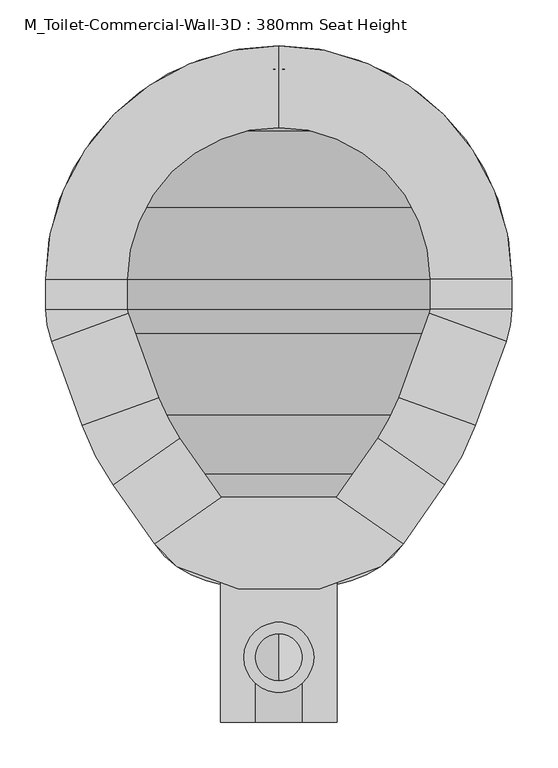
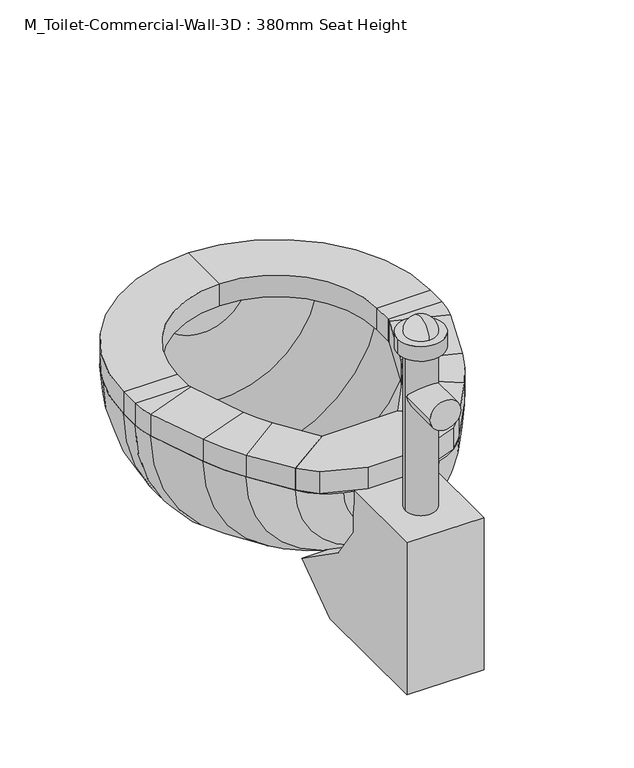
"""IFC4 building model written with IfcOpenShell, lengths in millimetres: flow terminal geometry, M_Toilet-Commercial-Wall-3D : 380mm Seat Height."""

from ifc_helpers import new_model, si_unit, point, frame, frame_2d, origin, place, context, project, spatial, polyline, circle_curve, ellipse_curve, trimmed, segment, composite_curve, outline, extrude, source, transform, mapped, element, save
from ifc_brep_helpers import plane_surface, cylinder_surface, revolved_surface, advanced_brep


def m_toilet_commercial_wall_3d_380mm_seat_height_fb359b30(model_context):
    return source(origin(), model_context, "Body", "SolidModel", [
        extrude(outline(polyline([(227.8037941, 341.9), (227.8037941, 268.296452), (271.5103185, 205.8770663), (375.5426282, 133.0328588), (295.0454017, 76.2), (75.0, 76.2), (75.0, 341.9), (227.8037941, 341.9)])), frame((341.4031538, 0.0, 0.0), z_axis=(1.0, 0.0, 0.0), x_axis=(0.0, 1.0, 0.0)), (0.0, 0.0, 1.0), 127.0),
        extrude(outline(composite_curve([segment(trimmed(circle_curve(frame_2d((404.9031538, 145.5352737)), 25.4), [point((379.5031538, 145.5352737))], [point((430.3031538, 145.5352737))], False, "CARTESIAN"), True, "CONTINUOUS"), segment(trimmed(circle_curve(frame_2d((404.9031538, 145.5352737)), 25.4), [point((430.3031538, 145.5352737))], [point((379.5031538, 145.5352737))], False, "CARTESIAN"), True, "CONTINUOUS")], self_intersect=False)), frame((0.0, 0.0, 341.9), z_axis=(0.0, 0.0, 1.0), x_axis=(1.0, 0.0, 0.0)), (0.0, 0.0, 1.0), 279.4),
        extrude(outline(composite_curve([segment(trimmed(circle_curve(frame_2d((543.2113641, 404.9031538)), 25.4), [point((543.2113641, 379.5031538))], [point((543.2113641, 430.3031538))], False, "CARTESIAN"), True, "CONTINUOUS"), segment(trimmed(circle_curve(frame_2d((543.2113641, 404.9031538)), 25.4), [point((543.2113641, 430.3031538))], [point((543.2113641, 379.5031538))], False, "CARTESIAN"), True, "CONTINUOUS")], self_intersect=False)), frame((0.0, 75.0, 0.0), z_axis=(0.0, 1.0, 0.0), x_axis=(0.0, 0.0, 1.0)), (0.0, 0.0, 1.0), 70.64375),
        extrude(outline(composite_curve([segment(trimmed(circle_curve(frame_2d((404.9031538, 145.5352737)), 38.1), [point((366.8031538, 145.5352737))], [point((443.0031538, 145.5352737))], False, "CARTESIAN"), True, "CONTINUOUS"), segment(trimmed(circle_curve(frame_2d((404.9031538, 145.5352737)), 38.1), [point((443.0031538, 145.5352737))], [point((366.8031538, 145.5352737))], False, "CARTESIAN"), True, "CONTINUOUS")], self_intersect=False)), frame((0.0, 0.0, 621.3), z_axis=(0.0, 0.0, 1.0), x_axis=(1.0, 0.0, 0.0)), (0.0, 0.0, 1.0), 25.4),
        advanced_brep(
        [(404.9031538, 119.9176912, 646.7), (404.9031538, 171.1528563, 646.7), (404.9031538, 145.5352737, 672.3175826), (404.9031538, 145.5352737, 646.7)],
        [
            (0, 1, circle_curve(frame((404.9031538, 145.5352737, 646.7), z_axis=(0.0, 0.0, 1.0), x_axis=(0.0, 1.0, 0.0)), 25.6175826)),
            (1, 2, circle_curve(frame((404.9031538, 145.5352737, 646.7), z_axis=(1.0, 0.0, 0.0), x_axis=(0.0, -1.0, 0.0)), 25.6175826)),
            (2, 0, circle_curve(frame((404.9031538, 145.5352737, 646.7), z_axis=(1.0, 0.0, 0.0), x_axis=(0.0, 1.0, 0.0)), 25.6175826)),
            (1, 0, circle_curve(frame((404.9031538, 145.5352737, 646.7), z_axis=(0.0, 0.0, 1.0), x_axis=(0.0, 1.0, 0.0)), 25.6175826)),
            (3, 1),
            (0, 3),
        ],
        [
            revolved_surface(trimmed(ellipse_curve(frame((404.9031538, 145.5352737, 646.7), z_axis=(-1.0, 0.0, 0.0), x_axis=(0.0, -1.0, 0.0)), 25.6175826, 25.6175826), [point((404.9031538, 145.5352737, 672.3175826))], [point((404.9031538, 171.1528563, 646.7))], True, "CARTESIAN"), (404.9031538, 145.5352737, 711.3277273), (0.0, 0.0, -1.0)),
            plane_surface(frame((404.9031538, 145.5352737, 646.7), z_axis=(0.0, 0.0, -1.0), x_axis=(0.0, 1.0, 0.0))),
        ],
        [
            (0, [[1, 2, 3]]),
            (0, [[4, -3, -2]]),
            (1, [[5, -1, 6]]),
            (1, [[-6, -4, -5]]),
        ],
    ),
        advanced_brep(
        [(491.7762702, 796.2819257, 341.9), (404.9031538, 811.6, 341.9), (404.9031538, 786.2, 341.9), (483.0889586, 772.4137331, 341.9), (566.547764, 719.2446102, 341.9), (619.7168869, 635.7858048, 341.9), (633.5031538, 557.6, 341.9), (633.5031538, 524.7148212, 341.9), (628.9077315, 498.6528863, 341.9), (596.6355667, 409.9858422, 341.9), (562.9565296, 345.2890139, 341.9), (525.0728964, 291.1855786, 341.9), (468.1430637, 251.3228806, 341.9), (404.9031538, 234.3777978, 341.9), (404.9031538, 208.0817829, 341.9), (483.6469009, 229.1811063, 341.9), (540.5767337, 269.0438043, 341.9), (585.6810159, 333.4593951, 341.9), (619.360053, 398.1562234, 341.9), (652.7759241, 489.9655747, 341.9), (658.9031538, 524.7148212, 341.9), (658.9031538, 557.6, 341.9), (643.5850795, 644.4731164, 341.9), (584.5082762, 737.2051224, 341.9), (318.0300374, 796.2819257, 341.9), (225.2980314, 737.2051224, 341.9), (166.2212281, 644.4731164, 341.9), (150.9031538, 557.6, 341.9), (150.9031538, 524.7148212, 341.9), (157.0303835, 489.9655747, 341.9), (190.4462546, 398.1562234, 341.9), (224.1252917, 333.4593951, 341.9), (269.229574, 269.0438043, 341.9), (326.1594067, 229.1811063, 341.9), (341.663244, 251.3228806, 341.9), (284.7334112, 291.1855786, 341.9), (246.849778, 345.2890139, 341.9), (213.1707409, 409.9858422, 341.9), (180.8985761, 498.6528863, 341.9), (176.3031538, 524.7148212, 341.9), (176.3031538, 557.6, 341.9), (190.0894207, 635.7858048, 341.9), (243.2585436, 719.2446102, 341.9), (326.7173491, 772.4137331, 341.9)],
        [
            (0, 1, circle_curve(frame((404.9031538, 557.6, 341.9), z_axis=(0.0, 0.0, 1.0), x_axis=(1.0, 0.0, 0.0)), 254.0)),
            (1, 2),
            (2, 3, circle_curve(frame((404.9031538, 557.6, 341.9), z_axis=(0.0, 0.0, -1.0), x_axis=(1.0, 0.0, 0.0)), 228.6)),
            (3, 4, circle_curve(frame((404.9031538, 557.6, 341.9), z_axis=(0.0, 0.0, -1.0), x_axis=(1.0, 0.0, 0.0)), 228.6)),
            (4, 5, circle_curve(frame((404.9031538, 557.6, 341.9), z_axis=(0.0, 0.0, -1.0), x_axis=(1.0, 0.0, 0.0)), 228.6)),
            (5, 6, circle_curve(frame((404.9031538, 557.6, 341.9), z_axis=(0.0, 0.0, -1.0), x_axis=(1.0, 0.0, 0.0)), 228.6)),
            (6, 7),
            (7, 8, circle_curve(frame((557.3031538, 524.7148212, 341.9), z_axis=(0.0, 0.0, -1.0), x_axis=(1.0, 0.0, 0.0)), 76.2)),
            (8, 9),
            (9, 10, circle_curve(frame((334.0854485, 505.5462703, 341.9), z_axis=(0.0, 0.0, -1.0), x_axis=(1.0, 0.0, 0.0)), 279.4)),
            (10, 11),
            (11, 12, circle_curve(frame((441.8470487, 349.4609446, 341.9), z_axis=(0.0, 0.0, -1.0), x_axis=(1.0, 0.0, 0.0)), 101.6)),
            (12, 13),
            (13, 14),
            (14, 15),
            (15, 16, circle_curve(frame((457.350886, 327.3191703, 341.9), z_axis=(0.0, 0.0, 1.0), x_axis=(1.0, 0.0, 0.0)), 101.6)),
            (16, 17),
            (17, 18, circle_curve(frame((356.8099347, 493.7166514, 341.9), z_axis=(0.0, 0.0, 1.0), x_axis=(1.0, 0.0, 0.0)), 279.4)),
            (18, 19),
            (19, 20, circle_curve(frame((557.3031538, 524.7148212, 341.9), z_axis=(0.0, 0.0, 1.0), x_axis=(1.0, 0.0, 0.0)), 101.6)),
            (20, 21),
            (21, 22, circle_curve(frame((404.9031538, 557.6, 341.9), z_axis=(0.0, 0.0, 1.0), x_axis=(1.0, 0.0, 0.0)), 254.0)),
            (22, 23, circle_curve(frame((404.9031538, 557.6, 341.9), z_axis=(0.0, 0.0, 1.0), x_axis=(1.0, 0.0, 0.0)), 254.0)),
            (23, 0, circle_curve(frame((404.9031538, 557.6, 341.9), z_axis=(0.0, 0.0, 1.0), x_axis=(1.0, 0.0, 0.0)), 254.0)),
            (24, 25, circle_curve(frame((404.9031538, 557.6, 341.9), z_axis=(0.0, 0.0, 1.0), x_axis=(-1.0, 0.0, 0.0)), 254.0)),
            (25, 26, circle_curve(frame((404.9031538, 557.6, 341.9), z_axis=(0.0, 0.0, 1.0), x_axis=(-1.0, 0.0, 0.0)), 254.0)),
            (26, 27, circle_curve(frame((404.9031538, 557.6, 341.9), z_axis=(0.0, 0.0, 1.0), x_axis=(-1.0, 0.0, 0.0)), 254.0)),
            (27, 28),
            (28, 29, circle_curve(frame((252.5031538, 524.7148212, 341.9), z_axis=(0.0, 0.0, 1.0), x_axis=(-1.0, 0.0, 0.0)), 101.6)),
            (29, 30),
            (30, 31, circle_curve(frame((452.9963729, 493.7166514, 341.9), z_axis=(0.0, 0.0, 1.0), x_axis=(-1.0, 0.0, 0.0)), 279.4)),
            (31, 32),
            (32, 33, circle_curve(frame((352.4554217, 327.3191703, 341.9), z_axis=(0.0, 0.0, 1.0), x_axis=(-1.0, 0.0, 0.0)), 101.6)),
            (33, 14),
            (13, 34),
            (34, 35, circle_curve(frame((367.9592589, 349.4609446, 341.9), z_axis=(0.0, 0.0, -1.0), x_axis=(-1.0, 0.0, 0.0)), 101.6)),
            (35, 36),
            (36, 37, circle_curve(frame((475.7208592, 505.5462703, 341.9), z_axis=(0.0, 0.0, -1.0), x_axis=(-1.0, 0.0, 0.0)), 279.4)),
            (37, 38),
            (38, 39, circle_curve(frame((252.5031538, 524.7148212, 341.9), z_axis=(0.0, 0.0, -1.0), x_axis=(-1.0, 0.0, 0.0)), 76.2)),
            (39, 40),
            (40, 41, circle_curve(frame((404.9031538, 557.6, 341.9), z_axis=(0.0, 0.0, -1.0), x_axis=(-1.0, 0.0, 0.0)), 228.6)),
            (41, 42, circle_curve(frame((404.9031538, 557.6, 341.9), z_axis=(0.0, 0.0, -1.0), x_axis=(-1.0, 0.0, 0.0)), 228.6)),
            (42, 43, circle_curve(frame((404.9031538, 557.6, 341.9), z_axis=(0.0, 0.0, -1.0), x_axis=(-1.0, 0.0, 0.0)), 228.6)),
            (43, 2, circle_curve(frame((404.9031538, 557.6, 341.9), z_axis=(0.0, 0.0, -1.0), x_axis=(-1.0, 0.0, 0.0)), 228.6)),
            (1, 24, circle_curve(frame((404.9031538, 557.6, 341.9), z_axis=(0.0, 0.0, 1.0), x_axis=(-1.0, 0.0, 0.0)), 254.0)),
            (0, 24, circle_curve(frame((404.9031538, 796.2819257, 341.9), z_axis=(0.0, 1.0, 0.0), x_axis=(1.0, 0.0, 0.0)), 86.8731164)),
            (43, 3, circle_curve(frame((404.9031538, 772.4137331, 341.9), z_axis=(0.0, -1.0, 0.0), x_axis=(1.0, 0.0, 0.0)), 78.1858048)),
            (42, 4, circle_curve(frame((404.9031538, 719.2446102, 341.9), z_axis=(0.0, -1.0, 0.0), x_axis=(1.0, 0.0, 0.0)), 161.6446102)),
            (41, 5, circle_curve(frame((404.9031538, 635.7858048, 341.9), z_axis=(0.0, -1.0, 0.0), x_axis=(1.0, 0.0, 0.0)), 214.8137331)),
            (40, 6, circle_curve(frame((404.9031538, 557.6, 341.9), z_axis=(0.0, -1.0, 0.0), x_axis=(1.0, 0.0, 0.0)), 228.6)),
            (39, 7, circle_curve(frame((404.9031538, 524.7148212, 341.9), z_axis=(0.0, -1.0, 0.0), x_axis=(1.0, 0.0, 0.0)), 228.6)),
            (38, 8, circle_curve(frame((404.9031538, 498.6528863, 341.9), z_axis=(0.0, -1.0, 0.0), x_axis=(1.0, 0.0, 0.0)), 224.0045777)),
            (37, 9, circle_curve(frame((404.9031538, 409.9858422, 341.9), z_axis=(0.0, -1.0, 0.0), x_axis=(1.0, 0.0, 0.0)), 191.7324129)),
            (36, 10, circle_curve(frame((404.9031538, 345.2890139, 341.9), z_axis=(0.0, -1.0, 0.0), x_axis=(1.0, 0.0, 0.0)), 158.0533758)),
            (35, 11, circle_curve(frame((404.9031538, 291.1855786, 341.9), z_axis=(0.0, -1.0, 0.0), x_axis=(1.0, 0.0, 0.0)), 120.1697426)),
            (34, 12, circle_curve(frame((404.9031538, 251.3228806, 341.9), z_axis=(0.0, -1.0, 0.0), x_axis=(1.0, 0.0, 0.0)), 63.2399099)),
            (33, 15, circle_curve(frame((404.9031538, 229.1811063, 341.9), z_axis=(0.0, -1.0, 0.0), x_axis=(1.0, 0.0, 0.0)), 78.7437471)),
            (32, 16, circle_curve(frame((404.9031538, 269.0438043, 341.9), z_axis=(0.0, -1.0, 0.0), x_axis=(1.0, 0.0, 0.0)), 135.6735798)),
            (31, 17, circle_curve(frame((404.9031538, 333.4593951, 341.9), z_axis=(0.0, -1.0, 0.0), x_axis=(1.0, 0.0, 0.0)), 180.7778621)),
            (30, 18, circle_curve(frame((404.9031538, 398.1562234, 341.9), z_axis=(0.0, -1.0, 0.0), x_axis=(1.0, 0.0, 0.0)), 214.4568992)),
            (29, 19, circle_curve(frame((404.9031538, 489.9655747, 341.9), z_axis=(0.0, -1.0, 0.0), x_axis=(1.0, 0.0, 0.0)), 247.8727703)),
            (28, 20, circle_curve(frame((404.9031538, 524.7148212, 341.9), z_axis=(0.0, -1.0, 0.0), x_axis=(1.0, 0.0, 0.0)), 254.0)),
            (27, 21, circle_curve(frame((404.9031538, 557.6, 341.9), z_axis=(0.0, -1.0, 0.0), x_axis=(1.0, 0.0, 0.0)), 254.0)),
            (26, 22, circle_curve(frame((404.9031538, 644.4731164, 341.9), z_axis=(0.0, -1.0, 0.0), x_axis=(1.0, 0.0, 0.0)), 238.6819257)),
            (25, 23, circle_curve(frame((404.9031538, 737.2051224, 341.9), z_axis=(0.0, -1.0, 0.0), x_axis=(1.0, 0.0, 0.0)), 179.6051224)),
        ],
        [
            plane_surface(frame((404.9031538, 916.8102448, 341.9), z_axis=(0.0, 0.0, 1.0), x_axis=(1.0, 0.0, 0.0))),
            plane_surface(frame((404.9031538, 916.8102448, 341.9), z_axis=(0.0, 0.0, 1.0), x_axis=(-1.0, 0.0, 0.0))),
            revolved_surface(trimmed(ellipse_curve(frame((404.9031538, 557.6, 341.9), z_axis=(0.0, 0.0, 1.0), x_axis=(1.0, 0.0, 0.0)), 254.0, 254.0), [point((491.7762702, 796.2819257, 341.9))], [point((404.9031538, 811.6, 341.9))], True, "CARTESIAN"), (404.9031538, 916.8102448, 341.9), (0.0, 1.0, 0.0)),
            revolved_surface(trimmed(ellipse_curve(frame((404.9031538, 557.6, 341.9), z_axis=(0.0, 0.0, -1.0), x_axis=(1.0, 0.0, 0.0)), 228.6, 228.6), [point((404.9031538, 786.2, 341.9))], [point((483.0889586, 772.4137331, 341.9))], True, "CARTESIAN"), (404.9031538, 916.8102448, 341.9), (0.0, 1.0, 0.0)),
            revolved_surface(trimmed(ellipse_curve(frame((404.9031538, 557.6, 341.9), z_axis=(0.0, 0.0, -1.0), x_axis=(1.0, 0.0, 0.0)), 228.6, 228.6), [point((483.0889586, 772.4137331, 341.9))], [point((566.547764, 719.2446102, 341.9))], True, "CARTESIAN"), (404.9031538, 916.8102448, 341.9), (0.0, 1.0, 0.0)),
            revolved_surface(trimmed(ellipse_curve(frame((404.9031538, 557.6, 341.9), z_axis=(0.0, 0.0, -1.0), x_axis=(1.0, 0.0, 0.0)), 228.6, 228.6), [point((566.547764, 719.2446102, 341.9))], [point((619.7168869, 635.7858048, 341.9))], True, "CARTESIAN"), (404.9031538, 916.8102448, 341.9), (0.0, 1.0, 0.0)),
            revolved_surface(trimmed(ellipse_curve(frame((404.9031538, 557.6, 341.9), z_axis=(0.0, 0.0, -1.0), x_axis=(1.0, 0.0, 0.0)), 228.6, 228.6), [point((619.7168869, 635.7858048, 341.9))], [point((633.5031538, 557.6, 341.9))], True, "CARTESIAN"), (404.9031538, 916.8102448, 341.9), (0.0, 1.0, 0.0)),
            revolved_surface(polyline([(633.5031538, 557.6, 341.9), (633.5031538, 524.7148212, 341.9)]), (404.9031538, 916.8102448, 341.9), (0.0, 1.0, 0.0)),
            revolved_surface(trimmed(ellipse_curve(frame((557.3031538, 524.7148212, 341.9), z_axis=(0.0, 0.0, -1.0), x_axis=(1.0, 0.0, 0.0)), 76.2, 76.2), [point((633.5031538, 524.7148212, 341.9))], [point((628.9077315, 498.6528863, 341.9))], True, "CARTESIAN"), (404.9031538, 916.8102448, 341.9), (0.0, 1.0, 0.0)),
            revolved_surface(polyline([(628.9077315, 498.6528863, 341.9), (596.6355667, 409.9858422, 341.9)]), (404.9031538, 916.8102448, 341.9), (0.0, 1.0, 0.0)),
            revolved_surface(trimmed(ellipse_curve(frame((334.0854485, 505.5462703, 341.9), z_axis=(0.0, 0.0, -1.0), x_axis=(1.0, 0.0, 0.0)), 279.4, 279.4), [point((596.6355667, 409.9858422, 341.9))], [point((562.9565296, 345.2890139, 341.9))], True, "CARTESIAN"), (404.9031538, 916.8102448, 341.9), (0.0, 1.0, 0.0)),
            revolved_surface(polyline([(562.9565296, 345.2890139, 341.9), (525.0728964, 291.1855786, 341.9)]), (404.9031538, 916.8102448, 341.9), (0.0, 1.0, 0.0)),
            revolved_surface(trimmed(ellipse_curve(frame((441.8470487, 349.4609446, 341.9), z_axis=(0.0, 0.0, -1.0), x_axis=(1.0, 0.0, 0.0)), 101.6, 101.6), [point((525.0728964, 291.1855786, 341.9))], [point((468.1430637, 251.3228806, 341.9))], True, "CARTESIAN"), (404.9031538, 916.8102448, 341.9), (0.0, 1.0, 0.0)),
            revolved_surface(polyline([(468.1430637, 251.3228806, 341.9), (404.9031538, 234.3777978, 341.9)]), (404.9031538, 916.8102448, 341.9), (0.0, 1.0, 0.0)),
            revolved_surface(polyline([(404.9031538, 208.0817829, 341.9), (483.6469009, 229.1811063, 341.9)]), (404.9031538, 916.8102448, 341.9), (0.0, 1.0, 0.0)),
            revolved_surface(trimmed(ellipse_curve(frame((457.350886, 327.3191703, 341.9), z_axis=(0.0, 0.0, 1.0), x_axis=(1.0, 0.0, 0.0)), 101.6, 101.6), [point((483.6469009, 229.1811063, 341.9))], [point((540.5767337, 269.0438043, 341.9))], True, "CARTESIAN"), (404.9031538, 916.8102448, 341.9), (0.0, 1.0, 0.0)),
            revolved_surface(polyline([(540.5767337, 269.0438043, 341.9), (585.6810159, 333.4593951, 341.9)]), (404.9031538, 916.8102448, 341.9), (0.0, 1.0, 0.0)),
            revolved_surface(trimmed(ellipse_curve(frame((356.8099347, 493.7166514, 341.9), z_axis=(0.0, 0.0, 1.0), x_axis=(1.0, 0.0, 0.0)), 279.4, 279.4), [point((585.6810159, 333.4593951, 341.9))], [point((619.360053, 398.1562234, 341.9))], True, "CARTESIAN"), (404.9031538, 916.8102448, 341.9), (0.0, 1.0, 0.0)),
            revolved_surface(polyline([(619.360053, 398.1562234, 341.9), (652.7759241, 489.9655747, 341.9)]), (404.9031538, 916.8102448, 341.9), (0.0, 1.0, 0.0)),
            revolved_surface(trimmed(ellipse_curve(frame((557.3031538, 524.7148212, 341.9), z_axis=(0.0, 0.0, 1.0), x_axis=(1.0, 0.0, 0.0)), 101.6, 101.6), [point((652.7759241, 489.9655747, 341.9))], [point((658.9031538, 524.7148212, 341.9))], True, "CARTESIAN"), (404.9031538, 916.8102448, 341.9), (0.0, 1.0, 0.0)),
            cylinder_surface(frame((404.9031538, 916.8102448, 341.9), z_axis=(0.0, 1.0, 0.0), x_axis=(1.0, 0.0, 0.0)), 254.0),
            revolved_surface(trimmed(ellipse_curve(frame((404.9031538, 557.6, 341.9), z_axis=(0.0, 0.0, 1.0), x_axis=(1.0, 0.0, 0.0)), 254.0, 254.0), [point((658.9031538, 557.6, 341.9))], [point((643.5850795, 644.4731164, 341.9))], True, "CARTESIAN"), (404.9031538, 916.8102448, 341.9), (0.0, 1.0, 0.0)),
            revolved_surface(trimmed(ellipse_curve(frame((404.9031538, 557.6, 341.9), z_axis=(0.0, 0.0, 1.0), x_axis=(1.0, 0.0, 0.0)), 254.0, 254.0), [point((643.5850795, 644.4731164, 341.9))], [point((584.5082762, 737.2051224, 341.9))], True, "CARTESIAN"), (404.9031538, 916.8102448, 341.9), (0.0, 1.0, 0.0)),
            revolved_surface(trimmed(ellipse_curve(frame((404.9031538, 557.6, 341.9), z_axis=(0.0, 0.0, 1.0), x_axis=(1.0, 0.0, 0.0)), 254.0, 254.0), [point((584.5082762, 737.2051224, 341.9))], [point((491.7762702, 796.2819257, 341.9))], True, "CARTESIAN"), (404.9031538, 916.8102448, 341.9), (0.0, 1.0, 0.0)),
        ],
        [
            (0, [[1, 2, 3, 4, 5, 6, 7, 8, 9, 10, 11, 12, 13, 14, 15, 16, 17, 18, 19, 20, 21, 22, 23, 24]]),
            (1, [[25, 26, 27, 28, 29, 30, 31, 32, 33, 34, -14, 35, 36, 37, 38, 39, 40, 41, 42, 43, 44, 45, -2, 46]]),
            (2, [[-1, 47, -46]]),
            (3, [[48, -3, -45]]),
            (4, [[49, -4, -48, -44]]),
            (5, [[50, -5, -49, -43]]),
            (6, [[51, -6, -50, -42]]),
            (7, [[52, -7, -51, -41]]),
            (8, [[53, -8, -52, -40]]),
            (9, [[54, -9, -53, -39]]),
            (10, [[55, -10, -54, -38]]),
            (11, [[56, -11, -55, -37]]),
            (12, [[57, -12, -56, -36]]),
            (13, [[-13, -57, -35]]),
            (14, [[58, -15, -34]]),
            (15, [[59, -16, -58, -33]]),
            (16, [[60, -17, -59, -32]]),
            (17, [[61, -18, -60, -31]]),
            (18, [[62, -19, -61, -30]]),
            (19, [[63, -20, -62, -29]]),
            (20, [[64, -21, -63, -28]]),
            (21, [[65, -22, -64, -27]]),
            (22, [[66, -23, -65, -26]]),
            (23, [[-47, -24, -66, -25]]),
        ],
    ),
        advanced_brep(
        [(467.7541169, 320.0347495, 341.9), (540.5767337, 269.0438043, 341.9), (540.5767337, 269.0438043, 380.0), (467.7541169, 320.0347495, 380.0), (512.8583992, 384.4503403, 341.9), (585.6810159, 333.4593951, 341.9), (585.6810159, 333.4593951, 380.0), (512.8583992, 384.4503403, 380.0), (619.360053, 398.1562234, 341.9), (535.821379, 428.5618141, 341.9), (619.360053, 398.1562234, 380.0), (535.821379, 428.5618141, 380.0), (569.2372501, 520.3711654, 341.9), (652.7759241, 489.9655747, 341.9), (652.7759241, 489.9655747, 380.0), (569.2372501, 520.3711654, 380.0), (658.9031538, 524.7148212, 341.9), (570.0031538, 524.7148212, 341.9), (658.9031538, 524.7148212, 380.0), (570.0031538, 524.7148212, 380.0), (570.0031538, 557.6, 341.9), (658.9031538, 557.6, 341.9), (658.9031538, 557.6, 380.0), (570.0031538, 557.6, 380.0), (404.9031538, 811.6, 341.9), (404.9031538, 722.7, 341.9), (404.9031538, 811.6, 380.0), (404.9031538, 722.7, 380.0), (150.9031538, 557.6, 341.9), (239.8031538, 557.6, 341.9), (150.9031538, 557.6, 380.0), (239.8031538, 557.6, 380.0), (239.8031538, 524.7148212, 341.9), (150.9031538, 524.7148212, 341.9), (150.9031538, 524.7148212, 380.0), (239.8031538, 524.7148212, 380.0), (157.0303835, 489.9655747, 341.9), (240.5690575, 520.3711654, 341.9), (157.0303835, 489.9655747, 380.0), (240.5690575, 520.3711654, 380.0), (273.9849286, 428.5618141, 341.9), (190.4462546, 398.1562234, 341.9), (190.4462546, 398.1562234, 380.0), (273.9849286, 428.5618141, 380.0), (224.1252917, 333.4593951, 341.9), (296.9479084, 384.4503403, 341.9), (224.1252917, 333.4593951, 380.0), (296.9479084, 384.4503403, 380.0), (342.0521907, 320.0347495, 341.9), (342.0521907, 320.0347495, 380.0), (269.229574, 269.0438043, 380.0), (269.229574, 269.0438043, 341.9)],
        [
            (0, 1),
            (1, 2),
            (2, 3),
            (3, 0),
            (0, 4),
            (4, 5),
            (5, 1),
            (5, 6),
            (6, 2),
            (6, 7),
            (7, 3),
            (7, 4),
            (8, 5, circle_curve(frame((356.8099347, 493.7166514, 341.9), z_axis=(0.0, 0.0, -1.0), x_axis=(0.819152044288991, -0.5735764363510472, 0.0)), 279.4)),
            (4, 9, circle_curve(frame((356.8099347, 493.7166514, 341.9), z_axis=(0.0, 0.0, 1.0), x_axis=(0.819152044288991, -0.5735764363510472, 0.0)), 190.5)),
            (9, 8),
            (10, 6, circle_curve(frame((356.8099347, 493.7166514, 380.0), z_axis=(0.0, 0.0, -1.0), x_axis=(0.819152044288991, -0.5735764363510472, 0.0)), 279.4)),
            (8, 10),
            (11, 7, circle_curve(frame((356.8099347, 493.7166514, 380.0), z_axis=(0.0, 0.0, -1.0), x_axis=(0.819152044288991, -0.5735764363510472, 0.0)), 190.5)),
            (10, 11),
            (11, 9),
            (9, 12),
            (12, 13),
            (13, 8),
            (13, 14),
            (14, 10),
            (14, 15),
            (15, 11),
            (15, 12),
            (16, 13, circle_curve(frame((557.3031538, 524.7148212, 341.9), z_axis=(0.0, 0.0, -1.0), x_axis=(0.93969262078591, -0.3420201433256644, 0.0)), 101.6)),
            (12, 17, circle_curve(frame((557.3031538, 524.7148212, 341.9), z_axis=(0.0, 0.0, 1.0), x_axis=(0.93969262078591, -0.3420201433256644, 0.0)), 12.7)),
            (17, 16),
            (18, 14, circle_curve(frame((557.3031538, 524.7148212, 380.0), z_axis=(0.0, 0.0, -1.0), x_axis=(0.93969262078591, -0.3420201433256644, 0.0)), 101.6)),
            (16, 18),
            (19, 15, circle_curve(frame((557.3031538, 524.7148212, 380.0), z_axis=(0.0, 0.0, -1.0), x_axis=(0.93969262078591, -0.3420201433256644, 0.0)), 12.7)),
            (18, 19),
            (19, 17),
            (17, 20),
            (20, 21),
            (21, 16),
            (21, 22),
            (22, 18),
            (22, 23),
            (23, 19),
            (23, 20),
            (24, 21, circle_curve(frame((404.9031538, 557.6, 341.9), z_axis=(0.0, 0.0, -1.0), x_axis=(1.0, 0.0, 0.0)), 254.0)),
            (20, 25, circle_curve(frame((404.9031538, 557.6, 341.9), z_axis=(0.0, 0.0, 1.0), x_axis=(1.0, 0.0, 0.0)), 165.1)),
            (25, 24),
            (26, 22, circle_curve(frame((404.9031538, 557.6, 380.0), z_axis=(0.0, 0.0, -1.0), x_axis=(1.0, 0.0, 0.0)), 254.0)),
            (24, 26),
            (27, 23, circle_curve(frame((404.9031538, 557.6, 380.0), z_axis=(0.0, 0.0, -1.0), x_axis=(1.0, 0.0, 0.0)), 165.1)),
            (26, 27),
            (27, 25),
            (28, 24, circle_curve(frame((404.9031538, 557.6, 341.9), z_axis=(0.0, 0.0, -1.0), x_axis=(0.0, 1.0, 0.0)), 254.0)),
            (25, 29, circle_curve(frame((404.9031538, 557.6, 341.9), z_axis=(0.0, 0.0, 1.0), x_axis=(0.0, 1.0, 0.0)), 165.1)),
            (29, 28),
            (30, 26, circle_curve(frame((404.9031538, 557.6, 380.0), z_axis=(0.0, 0.0, -1.0), x_axis=(0.0, 1.0, 0.0)), 254.0)),
            (28, 30),
            (31, 27, circle_curve(frame((404.9031538, 557.6, 380.0), z_axis=(0.0, 0.0, -1.0), x_axis=(0.0, 1.0, 0.0)), 165.1)),
            (30, 31),
            (31, 29),
            (29, 32),
            (32, 33),
            (33, 28),
            (33, 34),
            (34, 30),
            (34, 35),
            (35, 31),
            (35, 32),
            (36, 33, circle_curve(frame((252.5031538, 524.7148212, 341.9), z_axis=(0.0, 0.0, -1.0), x_axis=(-1.0, 0.0, 0.0)), 101.6)),
            (32, 37, circle_curve(frame((252.5031538, 524.7148212, 341.9), z_axis=(0.0, 0.0, 1.0), x_axis=(-1.0, 0.0, 0.0)), 12.7)),
            (37, 36),
            (38, 34, circle_curve(frame((252.5031538, 524.7148212, 380.0), z_axis=(0.0, 0.0, -1.0), x_axis=(-1.0, 0.0, 0.0)), 101.6)),
            (36, 38),
            (39, 35, circle_curve(frame((252.5031538, 524.7148212, 380.0), z_axis=(0.0, 0.0, -1.0), x_axis=(-1.0, 0.0, 0.0)), 12.7)),
            (38, 39),
            (39, 37),
            (37, 40),
            (40, 41),
            (41, 36),
            (41, 42),
            (42, 38),
            (42, 43),
            (43, 39),
            (43, 40),
            (44, 41, circle_curve(frame((452.9963729, 493.7166514, 341.9), z_axis=(0.0, 0.0, -1.0), x_axis=(-0.9396926207859084, -0.3420201433256685, 0.0)), 279.4)),
            (40, 45, circle_curve(frame((452.9963729, 493.7166514, 341.9), z_axis=(0.0, 0.0, 1.0), x_axis=(-0.9396926207859084, -0.3420201433256685, 0.0)), 190.5)),
            (45, 44),
            (46, 42, circle_curve(frame((452.9963729, 493.7166514, 380.0), z_axis=(0.0, 0.0, -1.0), x_axis=(-0.9396926207859084, -0.3420201433256685, 0.0)), 279.4)),
            (44, 46),
            (47, 43, circle_curve(frame((452.9963729, 493.7166514, 380.0), z_axis=(0.0, 0.0, -1.0), x_axis=(-0.9396926207859084, -0.3420201433256685, 0.0)), 190.5)),
            (46, 47),
            (47, 45),
            (48, 49),
            (49, 50),
            (50, 51),
            (51, 48),
            (45, 48),
            (51, 44),
            (50, 46),
            (49, 47),
        ],
        [
            plane_surface(frame((540.5767337, 269.0438043, 438.6203184), z_axis=(-0.5735764363510425, -0.8191520442889944, 0.0), x_axis=(0.8191520442889944, -0.5735764363510425, 0.0))),
            plane_surface(frame((467.7541169, 320.0347495, 341.9), z_axis=(0.0, 0.0, -1.0), x_axis=(0.5735764363510422, 0.8191520442889946, 0.0))),
            plane_surface(frame((540.5767337, 269.0438043, 341.9), z_axis=(0.8191520442889946, -0.5735764363510423, 0.0), x_axis=(0.5735764363510423, 0.8191520442889946, 0.0))),
            plane_surface(frame((540.5767337, 269.0438043, 380.0), z_axis=(0.0, 0.0, 1.0), x_axis=(0.5735764363510425, 0.8191520442889942, 0.0))),
            plane_surface(frame((467.7541169, 320.0347495, 380.0), z_axis=(-0.8191520442889942, 0.5735764363510425, 0.0), x_axis=(0.5735764363510425, 0.8191520442889942, 0.0))),
            plane_surface(frame((356.8099347, 493.7166514, 341.9), z_axis=(0.0, 0.0, -1.0), x_axis=(0.819152044288991, -0.5735764363510472, 0.0))),
            cylinder_surface(frame((356.8099347, 493.7166514, 341.9), z_axis=(0.0, 0.0, 1.0), x_axis=(0.819152044288991, -0.5735764363510472, 0.0)), 279.4),
            plane_surface(frame((356.8099347, 493.7166514, 380.0), z_axis=(0.0, 0.0, 1.0), x_axis=(0.819152044288991, -0.5735764363510472, 0.0))),
            revolved_surface(polyline([(512.8583991370527, 384.45034027512554, 380.0), (512.8583991370527, 384.45034027512554, 341.9)]), (356.8099347, 493.7166514, 341.9), (0.0, 0.0, 1.0)),
            plane_surface(frame((535.821379, 428.5618141, 341.9), z_axis=(0.0, 0.0, -1.0), x_axis=(0.34202014332565833, 0.9396926207859122, 0.0))),
            plane_surface(frame((619.360053, 398.1562234, 341.9), z_axis=(0.9396926207859126, -0.3420201433256572, 0.0), x_axis=(0.3420201433256572, 0.9396926207859126, 0.0))),
            plane_surface(frame((619.360053, 398.1562234, 380.0), z_axis=(0.0, 0.0, 1.0000000000000002), x_axis=(0.342020143325657, 0.9396926207859128, 0.0))),
            plane_surface(frame((535.821379, 428.5618141, 380.0), z_axis=(-0.9396926207859121, 0.342020143325659, 0.0), x_axis=(0.342020143325659, 0.9396926207859121, 0.0))),
            plane_surface(frame((557.3031538, 524.7148212, 341.9), z_axis=(0.0, 0.0, -1.0), x_axis=(0.93969262078591, -0.3420201433256644, 0.0))),
            cylinder_surface(frame((557.3031538, 524.7148212, 341.9), z_axis=(0.0, 0.0, 1.0), x_axis=(0.93969262078591, -0.3420201433256644, 0.0)), 101.6),
            plane_surface(frame((557.3031538, 524.7148212, 380.0), z_axis=(0.0, 0.0, 1.0), x_axis=(0.93969262078591, -0.3420201433256644, 0.0))),
            revolved_surface(polyline([(569.237250083981, 520.3711653797641, 380.0), (569.237250083981, 520.3711653797641, 341.9)]), (557.3031538, 524.7148212, 341.9), (0.0, 0.0, 1.0)),
            plane_surface(frame((570.0031538, 524.7148212, 341.9), z_axis=(0.0, 0.0, -1.0), x_axis=(0.0, 1.0, 0.0))),
            plane_surface(frame((658.9031538, 524.7148212, 341.9), z_axis=(1.0, 0.0, 0.0), x_axis=(0.0, 1.0, 0.0))),
            plane_surface(frame((658.9031538, 524.7148212, 380.0), z_axis=(0.0, 0.0, 1.0), x_axis=(0.0, 1.0, 0.0))),
            plane_surface(frame((570.0031538, 524.7148212, 380.0), z_axis=(-1.0, 0.0, 0.0), x_axis=(0.0, 1.0, 0.0))),
            plane_surface(frame((404.9031538, 557.6, 341.9), z_axis=(0.0, 0.0, -1.0), x_axis=(1.0, 0.0, 0.0))),
            cylinder_surface(frame((404.9031538, 557.6, 341.9), z_axis=(0.0, 0.0, 1.0), x_axis=(1.0, 0.0, 0.0)), 254.0),
            plane_surface(frame((404.9031538, 557.6, 380.0), z_axis=(0.0, 0.0, 1.0), x_axis=(1.0, 0.0, 0.0))),
            revolved_surface(polyline([(570.0031538, 557.6, 380.0), (570.0031538, 557.6, 341.9)]), (404.9031538, 557.6, 341.9), (0.0, 0.0, 1.0)),
            plane_surface(frame((404.9031538, 557.6, 341.9), z_axis=(0.0, 0.0, -1.0), x_axis=(0.0, 1.0, 0.0))),
            cylinder_surface(frame((404.9031538, 557.6, 341.9), z_axis=(0.0, 0.0, 1.0), x_axis=(0.0, 1.0, 0.0)), 254.0),
            plane_surface(frame((404.9031538, 557.6, 380.0), z_axis=(0.0, 0.0, 1.0), x_axis=(0.0, 1.0, 0.0))),
            revolved_surface(polyline([(404.9031538, 722.7, 380.0), (404.9031538, 722.7, 341.9)]), (404.9031538, 557.6, 341.9), (0.0, 0.0, 1.0)),
            plane_surface(frame((239.8031538, 557.6, 341.9), z_axis=(0.0, 0.0, -1.0), x_axis=(0.0, -1.0, 0.0))),
            plane_surface(frame((150.9031538, 557.6, 341.9), z_axis=(-1.0, 0.0, 0.0), x_axis=(0.0, -1.0, 0.0))),
            plane_surface(frame((150.9031538, 557.6, 380.0), z_axis=(0.0, 0.0, 1.0), x_axis=(0.0, -1.0, 0.0))),
            plane_surface(frame((239.8031538, 557.6, 380.0), z_axis=(1.0, 0.0, 0.0), x_axis=(0.0, -1.0, 0.0))),
            plane_surface(frame((252.5031538, 524.7148212, 341.9), z_axis=(0.0, 0.0, -1.0), x_axis=(-1.0, 0.0, 0.0))),
            cylinder_surface(frame((252.5031538, 524.7148212, 341.9), z_axis=(0.0, 0.0, 1.0), x_axis=(-1.0, 0.0, 0.0)), 101.6),
            plane_surface(frame((252.5031538, 524.7148212, 380.0), z_axis=(0.0, 0.0, 1.0), x_axis=(-1.0, 0.0, 0.0))),
            revolved_surface(polyline([(239.80315380000002, 524.7148212, 380.0), (239.80315380000002, 524.7148212, 341.9)]), (252.5031538, 524.7148212, 341.9), (0.0, 0.0, 1.0)),
            plane_surface(frame((240.5690575, 520.3711654, 341.9), z_axis=(0.0, 0.0, -1.0000000000000002), x_axis=(0.34202014332566893, -0.9396926207859084, 0.0))),
            plane_surface(frame((157.0303835, 489.9655747, 341.9), z_axis=(-0.9396926207859084, -0.3420201433256686, 0.0), x_axis=(0.3420201433256686, -0.9396926207859084, 0.0))),
            plane_surface(frame((157.0303835, 489.9655747, 380.0), z_axis=(0.0, 0.0, 1.0), x_axis=(0.3420201433256687, -0.9396926207859084, 0.0))),
            plane_surface(frame((240.5690575, 520.3711654, 380.0), z_axis=(0.9396926207859084, 0.3420201433256686, 0.0), x_axis=(0.3420201433256686, -0.9396926207859084, 0.0))),
            plane_surface(frame((452.9963729, 493.7166514, 341.9), z_axis=(0.0, 0.0, -1.0000000000000002), x_axis=(-0.9396926207859085, -0.34202014332566855, 0.0))),
            cylinder_surface(frame((452.9963729, 493.7166514, 341.9), z_axis=(0.0, 0.0, 1.0), x_axis=(-0.9396926207859084, -0.3420201433256685, 0.0)), 279.4),
            plane_surface(frame((452.9963729, 493.7166514, 380.0), z_axis=(0.0, 0.0, 1.0000000000000002), x_axis=(-0.9396926207859085, -0.34202014332566855, 0.0))),
            revolved_surface(polyline([(273.98492864028447, 428.5618140964601, 380.0), (273.98492864028447, 428.5618140964601, 341.9)]), (452.9963729, 493.7166514, 341.9), (0.0, 0.0, 1.0)),
            plane_surface(frame((269.229574, 269.0438043, 245.1796816), z_axis=(0.5735764363510472, -0.819152044288991, 0.0), x_axis=(0.819152044288991, 0.5735764363510472, 0.0))),
            plane_surface(frame((296.9479084, 384.4503403, 341.9), z_axis=(0.0, 0.0, -1.0), x_axis=(0.573576436351047, -0.8191520442889911, 0.0))),
            plane_surface(frame((224.1252917, 333.4593951, 341.9), z_axis=(-0.819152044288991, -0.5735764363510473, 0.0), x_axis=(0.5735764363510473, -0.819152044288991, 0.0))),
            plane_surface(frame((224.1252917, 333.4593951, 380.0), z_axis=(0.0, 0.0, 1.0), x_axis=(0.5735764363510477, -0.8191520442889907, 0.0))),
            plane_surface(frame((296.9479084, 384.4503403, 380.0), z_axis=(0.8191520442889914, 0.5735764363510468, 0.0), x_axis=(0.5735764363510468, -0.8191520442889914, 0.0))),
        ],
        [
            (0, [[1, 2, 3, 4]]),
            (1, [[-1, 5, 6, 7]]),
            (2, [[-2, -7, 8, 9]]),
            (3, [[-3, -9, 10, 11]]),
            (4, [[-4, -11, 12, -5]]),
            (5, [[13, -6, 14, 15]]),
            (6, [[16, -8, -13, 17]]),
            (7, [[18, -10, -16, 19]]),
            (8, [[-14, -12, -18, 20]]),
            (9, [[-15, 21, 22, 23]]),
            (10, [[-17, -23, 24, 25]]),
            (11, [[-19, -25, 26, 27]]),
            (12, [[-20, -27, 28, -21]]),
            (13, [[29, -22, 30, 31]]),
            (14, [[32, -24, -29, 33]]),
            (15, [[34, -26, -32, 35]]),
            (16, [[-30, -28, -34, 36]]),
            (17, [[-31, 37, 38, 39]]),
            (18, [[-33, -39, 40, 41]]),
            (19, [[-35, -41, 42, 43]]),
            (20, [[-36, -43, 44, -37]]),
            (21, [[45, -38, 46, 47]]),
            (22, [[48, -40, -45, 49]]),
            (23, [[50, -42, -48, 51]]),
            (24, [[-46, -44, -50, 52]]),
            (25, [[53, -47, 54, 55]]),
            (26, [[56, -49, -53, 57]]),
            (27, [[58, -51, -56, 59]]),
            (28, [[-54, -52, -58, 60]]),
            (29, [[-55, 61, 62, 63]]),
            (30, [[-57, -63, 64, 65]]),
            (31, [[-59, -65, 66, 67]]),
            (32, [[-60, -67, 68, -61]]),
            (33, [[69, -62, 70, 71]]),
            (34, [[72, -64, -69, 73]]),
            (35, [[74, -66, -72, 75]]),
            (36, [[-70, -68, -74, 76]]),
            (37, [[-71, 77, 78, 79]]),
            (38, [[-73, -79, 80, 81]]),
            (39, [[-75, -81, 82, 83]]),
            (40, [[-76, -83, 84, -77]]),
            (41, [[85, -78, 86, 87]]),
            (42, [[88, -80, -85, 89]]),
            (43, [[90, -82, -88, 91]]),
            (44, [[-86, -84, -90, 92]]),
            (45, [[93, 94, 95, 96]]),
            (46, [[-87, 97, -96, 98]]),
            (47, [[-89, -98, -95, 99]]),
            (48, [[-91, -99, -94, 100]]),
            (49, [[-92, -100, -93, -97]]),
        ],
    ),
        extrude(outline(polyline([(467.7541169, 320.0347495), (540.5767337, 269.0438043), (515.6262519, 244.0933226), (449.563909, 220.0485961), (360.2423986, 220.0485961), (294.1800557, 244.0933226), (269.229574, 269.0438043), (342.0521907, 320.0347495), (467.7541169, 320.0347495)])), frame((0.0, 0.0, 341.9), z_axis=(0.0, 0.0, 1.0), x_axis=(1.0, 0.0, 0.0)), (0.0, 0.0, 1.0), 38.1),
    ])


if __name__ == "__main__":
    model = new_model("IFC4")
    model_context = context("Model", 3, world=origin())
    ifc_project = project(units=[si_unit("LENGTHUNIT", "METRE", prefix="MILLI")], contexts=[model_context])
    site = spatial("IfcSite", under=ifc_project)
    building = spatial("IfcBuilding", under=site)
    placement = place(None, origin())
    m_toilet_commercial_wall_3d_380mm_seat_height_shape = m_toilet_commercial_wall_3d_380mm_seat_height_fb359b30(model_context)
    element("IfcFlowTerminal", 1, ObjectType="M_Toilet-Commercial-Wall-3D : 380mm Seat Height", at=placement, inside=building, context=model_context, shape_type="MappedRepresentation", body=[
        mapped(m_toilet_commercial_wall_3d_380mm_seat_height_shape, transform((0.0, 0.0, 0.0), x_axis=(1.0, 0.0, 0.0), y_axis=(0.0, 1.0, 0.0), z_axis=(0.0, 0.0, 1.0))),
    ])
    save(model, "model.ifc")

# Revit data of these elements
# Type "M_Toilet-Commercial-Wall-3D : 380mm Seat Height"
#   Mounting Height = 380 mm
#   Piping Material = Steel, Polished
#   Bowl Material = Porcelain, Ivory
#   Seat Material = Laminate, Ivory, Matte
#   Default Elevation = 0
# Element 1 (IfcFlowTerminal, "M_Toilet-Commercial-Wall-3D : 380mm Seat Height")
#   Materials on its faces: "Laminate, Ivory, Matte", "Porcelain, Ivory", "Steel, Polished"
# Materials
#   "Steel, Polished": class "Metal", colour RGB 57 57 57, transparency 0, Description = "Polished steel", Cost = 0
#   "Porcelain, Ivory": class "Ceramic", colour RGB 247 247 239, transparency 0, Description = "Porcelain, ivory", Cost = 0
#   "Laminate, Ivory, Matte": class "Plastic", colour RGB 247 247 239, transparency 0, Description = "Plastic Laminate - Ivory, Matte", Cost = 0
